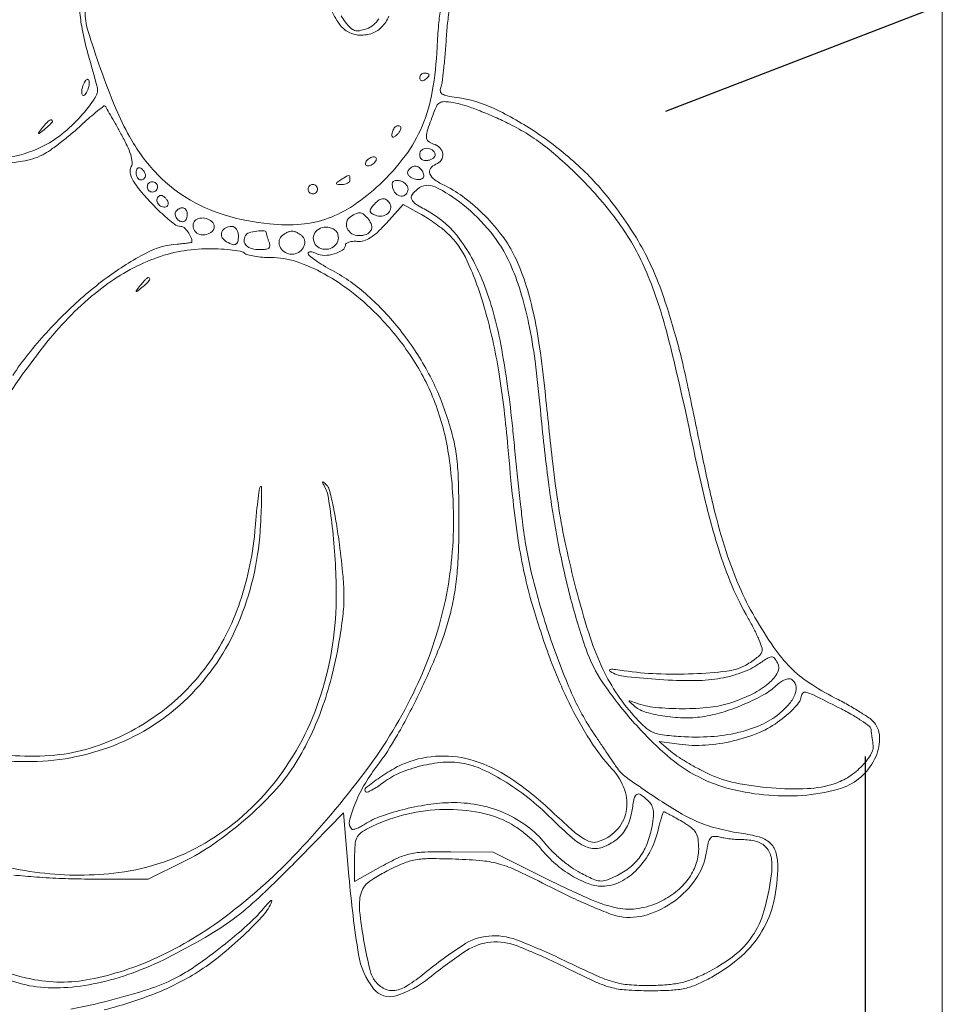
# Model space of a CAD drawing. Units: inches. Extents: x 2656 to 9931, y 1941 to 3068.
# Tile 35 of 46: x 2854 to 2868, y 2952 to 2967. Entities that reach past the tile are written whole.
import ezdxf

# ---------------------------------------------------------------- set-up
doc = ezdxf.new("R2010")
doc.units = ezdxf.units.IN
for name, color, linetype, lineweight in [('A-ANNO-DIMS', 2, 'Continuous', 18), ('A-ELEV-FNSH', 8, 'Continuous', 13), ('A-ELEV-ORN', 8, 'Continuous', 13)]:
    doc.layers.add(name, color=color, linetype=linetype, lineweight=lineweight)
doc.styles.get("Standard").update_dxf_attribs({"font": 'arial.ttf'})
doc.dimstyles.new('ISO-25', dxfattribs={"dimtxt": 6, "dimasz": 2.5, "dimexe": 1.25, "dimexo": 0.625, "dimtad": 1, "dimdec": 0, "dimlunit": 3, "dimtxsty": 'Standard', "dimcen": 2.5, "dimadec": 0, "dimazin": 0, "dimtfac": 1, "dimtdec": 0, "dimtmove": 0, "dimatfit": 3, "dimfxl": 1, "dimarcsym": 0})

# ---------------------------------------------------------------- blocks, each defined once
blk = doc.blocks.new('*D151')
at = {"layer": 'A-ANNO-DIMS', "color": 0, "lineweight": -2, "transparency": 16777216}
for p, q in [((2829.546, 2956.424), (2829.546, 2703.709)), ((2867.059, 2955.98), (2867.059, 2703.709)), ((2832.046, 2704.959), (2864.559, 2704.959))]:
    blk.add_line(p, q, dxfattribs=at)
at = {"layer": 'A-ANNO-DIMS', "color": 0, "transparency": 16777216}
for points in [[(2832.046, 2705.376), (2832.046, 2704.543), (2829.546, 2704.959)], [(2864.559, 2705.376), (2864.559, 2704.543), (2867.059, 2704.959)]]:
    blk.add_solid(points, dxfattribs=at)
at = {"layer": 'Defpoints', "color": 0, "transparency": 16777216}
for p in [(2829.546, 2957.049), (2867.059, 2956.605), (2867.059, 2704.959)]:
    blk.add_point(p, dxfattribs=at)
at = {"layer": 'A-ANNO-DIMS', "color": 0, "transparency": 16777216, "insert": (2848.302, 2708.689), "char_height": 6, "attachment_point": 5}
blk.add_mtext('3\'-1 1/2"', dxfattribs=at)
blk = doc.blocks.new('*D166')
at = {"layer": 'A-ANNO-DIMS', "color": 0, "lineweight": -2, "transparency": 16777216}
for p, q in [((2884.455, 2990.075), (2890.436, 2974.616)), ((2876.883, 2987.145), (2882.863, 2971.687)), ((2887.653, 2974.88), (2884.744, 2973.755)), ((2882.412, 2972.852), (2864.04, 2965.744))]:
    blk.add_line(p, q, dxfattribs=at)
at = {"layer": 'A-ANNO-DIMS', "color": 0, "transparency": 16777216}
for points in [[(2887.503, 2975.269), (2887.803, 2974.491), (2889.985, 2975.782)], [(2884.594, 2974.143), (2884.894, 2973.366), (2882.412, 2972.852)]]:
    blk.add_solid(points, dxfattribs=at)
at = {"layer": 'Defpoints', "color": 0, "transparency": 16777216}
for p in [(2884.229, 2990.658), (2876.657, 2987.728), (2882.412, 2972.852)]:
    blk.add_point(p, dxfattribs=at)
at = {"layer": 'A-ANNO-DIMS', "color": 0, "transparency": 16777216, "insert": (2870.73, 2972.287), "char_height": 6, "attachment_point": 5, "rotation": 21.1508}
blk.add_mtext('0\'-8"', dxfattribs=at)

msp = doc.modelspace()

# ---------------------------------------------------------------- linework, layer by layer
at = {"layer": 'A-ELEV-FNSH'}
msp.add_lwpolyline([(2826.64, 2994.347), (2868.226, 2994.347), (2868.226, 2892.035), (2826.64, 2892.035)], close=True, dxfattribs=at)
at = {"layer": 'A-ELEV-ORN'}
for points in [[(2855.174, 2967.3, 0.028596), (2855.206, 2967.037, 0.019917), (2855.288, 2966.67, 0.006616), (2855.436, 2966.14, -0.21756), (2855.409, 2965.955, -0.040075), (2855.195, 2965.675, -0.041303), (2854.904, 2965.4, -0.056735), (2854.6, 2965.209, -0.074881), (2854.055, 2965.042, -0.054125)], [(2854.109, 2952.6, 0.063438), (2854.524, 2952.497, 0.048495), (2854.996, 2952.487, 0.037857), (2855.505, 2952.565, 0.034879), (2856.037, 2952.728, 0.028198), (2856.582, 2952.973, 0.013653), (2857.141, 2953.284, 0.030316), (2857.545, 2953.557, 0.026779), (2857.942, 2953.897, 0.008593), (2858.495, 2954.443), (2859.166, 2955.13), (2859.249, 2954.169, 0.017456), (2859.394, 2952.984, 0.128416), (2859.621, 2952.466, 0.311108), (2859.962, 2952.36, 0.095606), (2860.463, 2952.63, -0.025392), (2861.026, 2953.043, -0.124698), (2861.396, 2953.172, -0.116398), (2861.795, 2953.114, -0.020849), (2862.488, 2952.806, 0.006689), (2862.954, 2952.582, 0.039752), (2863.207, 2952.488, 0.052181), (2863.442, 2952.448, 0.016514), (2863.798, 2952.436, 0.012108), (2864.123, 2952.444, 0.04207), (2864.331, 2952.472, 0.049914), (2864.513, 2952.531, 0.022452), (2864.737, 2952.643, 0.054702), (2865.187, 2952.96, 0.078378), (2865.497, 2953.336, 0.078505), (2865.676, 2953.788, 0.05507), (2865.736, 2954.334, 0.073105), (2865.706, 2954.537, 0.14057), (2865.618, 2954.674, 0.111241), (2865.454, 2954.764, 0.036328), (2865.182, 2954.82, -0.017364), (2865.028, 2954.846, -0.011942), (2864.854, 2954.885, -0.012054), (2864.69, 2954.932, -0.023906), (2864.562, 2954.978, -0.035914), (2864.252, 2955.133, -0.013112), (2863.836, 2955.395, -0.010281), (2863.442, 2955.67, -0.087803), (2863.294, 2955.825, 0.00053), (2863.245, 2955.897, 0.000109), (2863.16, 2956.023, 0.000114), (2863.061, 2956.171, 0.000108), (2862.959, 2956.321, -0.045796), (2862.618, 2956.942, -0.021393), (2862.287, 2957.8, -0.021231), (2862.02, 2958.719, -0.0319), (2861.874, 2959.54, -0.001287), (2861.841, 2959.838, -0.000643), (2861.801, 2960.214, -0.000639), (2861.76, 2960.604, -0.000943), (2861.726, 2960.947, 0.020553), (2861.546, 2962.22, 0.04686), (2861.284, 2963.153, 0.064624), (2860.927, 2963.81, 0.108526), (2860.461, 2964.226, -0.013252), (2860.262, 2964.345, -0.1368), (2860.198, 2964.415, -0.28166), (2860.204, 2964.483, -0.060529), (2860.288, 2964.572, -0.292683), (2860.552, 2964.604, -0.058258), (2860.972, 2964.339, -0.052773), (2861.394, 2963.918, -0.064866), (2861.686, 2963.444, -0.030734), (2861.844, 2963.023, -0.02351), (2861.967, 2962.546, -0.019015), (2862.065, 2961.967, -0.009465), (2862.146, 2961.228, 0.00962), (2862.266, 2960.142, 0.014652), (2862.416, 2959.206, 0.016506), (2862.603, 2958.374, 0.019831), (2862.836, 2957.606, 0.066026), (2863.091, 2957.098, 0.031307), (2863.541, 2956.518, 0.031311), (2864.062, 2955.996, 0.063647), (2864.54, 2955.672, 0.055485), (2865.032, 2955.488, 0.042522), (2865.599, 2955.395, 0.042331), (2866.177, 2955.399, 0.053334), (2866.701, 2955.504, 0.104768), (2866.992, 2955.669, 0.096785), (2867.202, 2955.942, 0.109583), (2867.278, 2956.245, 0.172667), (2867.195, 2956.497, 0.078073), (2867.133, 2956.555, 0.010534), (2866.983, 2956.654, 0.01194), (2866.799, 2956.763, 0.009802), (2866.597, 2956.871, -0.028546), (2866.213, 2957.096, -0.050975), (2865.93, 2957.328, -0.045238), (2865.679, 2957.631, -0.017925), (2865.39, 2958.088, -0.030624), (2865.156, 2958.552, -0.023473), (2864.956, 2959.083, -0.018746), (2864.771, 2959.74, -0.008967), (2864.581, 2960.595, 0.001102), (2864.391, 2961.515, 0.006759), (2864.285, 2961.988, 0.011262), (2864.191, 2962.348, 0.007165), (2864.067, 2962.762, 0.018233), (2863.907, 2963.21, 0.025477), (2863.729, 2963.597, 0.025141), (2863.511, 2963.968, 0.017087), (2863.228, 2964.368, 0.044384), (2862.72, 2964.925, 0.037111), (2862.093, 2965.421, 0.038623), (2861.444, 2965.79, 0.076899), (2860.879, 2965.957, -0.016318), (2860.734, 2965.981, -0.091012), (2860.661, 2966.01, -0.208145), (2860.633, 2966.051, -0.140788), (2860.638, 2966.109, 0.059531), (2860.657, 2966.183, 0.005389), (2860.681, 2966.375, 0.006933), (2860.703, 2966.604, 0.005366), (2860.722, 2966.855, -0.012637), (2860.744, 2967.112, -0.013655), (2860.78, 2967.361, -0.013252)], [(2860.639, 2967.314, 0.023375), (2860.606, 2967.062, 0.009261), (2860.583, 2966.714, -0.031116), (2860.51, 2966.049, -0.056426), (2860.356, 2965.523, -0.061102), (2860.1, 2965.074, -0.043729), (2859.714, 2964.642, -0.039093), (2859.318, 2964.324, -0.06347), (2858.935, 2964.129, -0.065711), (2858.524, 2964.039, -0.045332), (2858.048, 2964.043, -0.049376), (2857.363, 2964.18, -0.065569), (2856.785, 2964.443, -0.067894), (2856.31, 2964.838, -0.058197), (2855.929, 2965.366, -0.029232), (2855.719, 2965.799, -0.012926), (2855.492, 2966.391, -0.010579), (2855.3, 2966.971, -0.074704), (2855.256, 2967.264, -0.0517)], [(2858.97, 2967.304, 0.041294), (2859.105, 2967.067, 0.109032), (2859.227, 2966.955, 0.109354), (2859.384, 2966.903, 0.099066), (2859.581, 2966.923, 0.120027), (2859.739, 2967.018, 0.102309), (2859.854, 2967.189, 0.057096)], [(2859.7, 2967.146, -0.082559), (2859.62, 2967.056, -0.084337), (2859.515, 2966.998, -0.038037), (2859.407, 2966.968, -0.127103), (2859.335, 2966.973, -0.11952), (2859.271, 2967.012, -0.031788), (2859.191, 2967.103, -0.033217), (2859.132, 2967.192, -0.013391)], [(2853.796, 2964.937, 0.021823), (2854.311, 2964.991, 0.083985), (2854.616, 2965.091, 0.031152), (2854.732, 2965.161, 0.011426), (2854.886, 2965.274, 0.011275), (2855.049, 2965.405, 0.013273), (2855.198, 2965.537, -0.007108), (2855.33, 2965.657, -0.011939), (2855.446, 2965.754, -0.005638), (2855.543, 2965.83, -0.413391), (2855.561, 2965.828, -0.034188), (2855.576, 2965.806, -0.000712), (2855.64, 2965.693, -0.001658), (2855.715, 2965.561, -0.001115), (2855.799, 2965.409, -0.014931), (2855.892, 2965.228, -0.035606), (2855.947, 2965.088, -0.049197), (2855.97, 2964.981, -0.155471), (2855.955, 2964.911, 0.120552), (2855.939, 2964.851, 0.082364), (2855.948, 2964.78, 0.06067), (2855.985, 2964.698, 0.029026), (2856.05, 2964.602, 0.022485), (2856.228, 2964.391, 0.021702), (2856.426, 2964.195, 0.01756), (2856.61, 2964.039, 0.16831), (2856.706, 2964.006, -0.187338), (2856.757, 2963.987, -0.053599), (2856.814, 2963.922, -0.052999), (2856.859, 2963.842, -0.101355), (2856.874, 2963.769, -0.369146), (2856.868, 2963.763, -0.003978), (2856.808, 2963.754, -0.010014), (2856.737, 2963.745, -0.006066), (2856.652, 2963.738, 0.102377), (2856.179, 2963.602, 0.038016), (2855.589, 2963.232, 0.034625), (2854.97, 2962.705, 0.029805), (2854.396, 2962.072, 0.025999), (2854.163, 2961.749, 0.003163)], [(2853.875, 2961.115, -0.028373), (2854.681, 2962.254, -0.056082), (2855.463, 2963.036, -0.071786), (2856.251, 2963.498, -0.092393), (2857.071, 2963.666, -0.013431), (2857.27, 2963.665, -0.017308), (2857.452, 2963.652, -0.015196), (2857.601, 2963.632, -0.126503), (2857.663, 2963.604, 0.101758), (2857.717, 2963.577, 0.023151), (2857.819, 2963.554, 0.023036), (2857.942, 2963.539, 0.020609), (2858.069, 2963.534, -0.081277), (2858.449, 2963.474, -0.046227), (2858.875, 2963.287, -0.041516), (2859.312, 2962.996, -0.034768), (2859.724, 2962.62, -0.047065), (2860.226, 2961.981, -0.056002), (2860.567, 2961.294, -0.052207), (2860.763, 2960.51, -0.033786), (2860.831, 2959.575, -0.05658), (2860.69, 2958.266, -0.055783), (2860.258, 2957.014, -0.04941), (2859.505, 2955.766, -0.030886), (2858.401, 2954.463, -0.039889), (2857.397, 2953.571, -0.052556), (2856.348, 2952.94, -0.060616), (2855.335, 2952.61, -0.099916), (2854.437, 2952.614, -0.051733), (2853.786, 2952.82, -0.039695)], [(2854.178, 2954.187, 0.008256), (2854.522, 2954.157, 0.008262), (2854.912, 2954.135, 0.008791), (2855.295, 2954.127), (2856.213, 2954.124), (2856.741, 2954.385, 0.037754), (2857.203, 2954.659, 0.026153), (2857.682, 2955.032, 0.026418), (2858.109, 2955.444, 0.045079), (2858.414, 2955.836, 0.028905), (2858.644, 2956.245, 0.02616), (2858.835, 2956.692, 0.024873), (2858.985, 2957.179, 0.020872), (2859.098, 2957.707, 0.011221), (2859.156, 2958.106, 0.029314), (2859.174, 2958.396, 0.025822), (2859.16, 2958.705, 0.00712), (2859.105, 2959.189, 0.00881), (2859.059, 2959.509, 0.012431), (2859.006, 2959.792, 0.008644), (2858.952, 2960.024, 0.14575), (2858.912, 2960.091, 0.005212), (2858.864, 2960.133, 0.236159), (2858.852, 2960.137, 0.498193), (2858.848, 2960.129, 0.008614), (2858.874, 2960.083, -0.089875), (2858.939, 2959.894, -0.011245), (2858.997, 2959.464, -0.013414), (2859.04, 2958.961, -0.012898), (2859.057, 2958.45, -0.078199), (2858.825, 2956.917, -0.089178), (2858.136, 2955.605, -0.094631), (2857.073, 2954.672, -0.101406), (2855.766, 2954.225, -0.06271), (2854.574, 2954.222, -0.059511), (2853.396, 2954.512, -0.061335)], [(2854.024, 2955.915, 0.013073), (2854.359, 2955.904, 0.095042), (2855.696, 2956.15, 0.101899), (2856.811, 2956.872, 0.098684), (2857.574, 2957.997, 0.08367), (2857.906, 2959.398, 0.004935), (2857.92, 2959.655, 0.008259), (2857.927, 2959.871, 0.002726), (2857.928, 2960.054, 0.414775), (2857.915, 2960.068, 0.371773), (2857.899, 2960.054, 0.003199), (2857.876, 2959.889, 0.008961), (2857.853, 2959.692, 0.005421), (2857.832, 2959.459, -0.062277), (2857.6, 2958.319, -0.076581), (2857.101, 2957.356, -0.079646), (2856.354, 2956.616, -0.0747), (2855.397, 2956.127, -0.053032), (2854.872, 2956.011, -0.038092), (2854.272, 2955.99, -0.038832), (2853.696, 2956.059, -0.070977)], [(2855.548, 2952.148, 0.033055), (2856.284, 2952.381, 0.043026), (2856.918, 2952.694, 0.031455), (2857.248, 2952.924, 0.018917), (2857.611, 2953.235, 0.017394), (2857.928, 2953.549, 0.078159), (2858.074, 2953.763, 0.114181), (2858.081, 2953.795, 0.599459), (2858.069, 2953.802, 0.059878), (2858.025, 2953.763, 0.010894), (2857.955, 2953.682, -0.039265), (2857.711, 2953.427, -0.0147), (2857.331, 2953.109, -0.014829), (2856.93, 2952.811, -0.035002), (2856.61, 2952.62, -0.03988), (2856.209, 2952.456, -0.015079), (2855.626, 2952.288, -0.01477), (2855.041, 2952.158, -0.047431)]]:
    msp.add_lwpolyline(points, format="xyb", dxfattribs=at)
for points in [[(2855.228, 2966.144, 0.033304), (2855.213, 2966.096, 0.041541), (2855.206, 2966.05, 0.04665), (2855.207, 2966.012, 0.168083), (2855.218, 2965.991, 0.291964), (2855.235, 2965.987, 0.11331), (2855.256, 2966.001, 0.066301), (2855.278, 2966.031, 0.03436), (2855.298, 2966.074, 0.033304), (2855.313, 2966.122, 0.041541), (2855.32, 2966.168, 0.04665), (2855.319, 2966.206, 0.168083), (2855.309, 2966.228, 0.291964), (2855.292, 2966.232, 0.11331), (2855.27, 2966.218, 0.066301), (2855.248, 2966.187, 0.03436)], [(2860.32, 2966.253, 0.108972), (2860.326, 2966.228, 0.182303), (2860.341, 2966.213, 0.161196), (2860.364, 2966.211, 0.082592), (2860.39, 2966.222, 0.029505), (2860.417, 2966.241, 0.035638), (2860.44, 2966.262, 0.038439), (2860.456, 2966.282, 0.151918), (2860.461, 2966.296, 0.210953), (2860.456, 2966.308, 0.081139), (2860.44, 2966.318, 0.061769), (2860.417, 2966.325, 0.042167), (2860.39, 2966.327, 0.105053), (2860.364, 2966.322, 0.099167), (2860.341, 2966.305, 0.09642), (2860.325, 2966.281, 0.093332)], [(2861.648, 2965.571, -0.02318), (2861.924, 2965.42, -0.024394), (2862.179, 2965.246, -0.021618), (2862.441, 2965.03, -0.012473), (2862.739, 2964.749, -0.039784), (2863.327, 2964.063, -0.054855), (2863.73, 2963.359, -0.039702), (2864.051, 2962.425, -0.011344), (2864.399, 2960.931, 0.006591), (2864.634, 2959.877, 0.017333), (2864.839, 2959.13, 0.02365), (2865.047, 2958.558, 0.033029), (2865.29, 2958.071, -0.014848), (2865.38, 2957.905, -0.020336), (2865.451, 2957.751, -0.017573), (2865.498, 2957.622, -0.172671), (2865.497, 2957.564, -0.10754), (2865.469, 2957.521, -0.026105), (2865.405, 2957.465, -0.025574), (2865.322, 2957.406, -0.022994), (2865.232, 2957.354, -0.091881), (2864.964, 2957.273, -0.017748), (2864.458, 2957.234, -0.019702), (2863.902, 2957.234, -0.028696), (2863.415, 2957.281, 0.009481), (2863.282, 2957.299, 0.047771), (2863.208, 2957.301, 0.368655), (2863.193, 2957.286, 0.282694), (2863.204, 2957.266, 0.108907), (2863.401, 2957.197, 0.011453), (2863.888, 2957.151, 0.015255), (2864.397, 2957.13, 0.03383), (2864.785, 2957.152, 0.026779), (2864.958, 2957.183, 0.023197), (2865.136, 2957.233, 0.024046), (2865.297, 2957.296, 0.044005), (2865.421, 2957.365, -0.008574), (2865.576, 2957.467, -0.115161), (2865.64, 2957.489, -0.24786), (2865.685, 2957.47, -0.052764), (2865.734, 2957.398, -0.252743), (2865.734, 2957.255, -0.09163), (2865.602, 2957.092, -0.061736), (2865.357, 2956.931, -0.0348), (2865.029, 2956.796, -0.05395), (2864.712, 2956.727, -0.025613), (2864.295, 2956.705, -0.025459), (2863.884, 2956.725, -0.063366), (2863.591, 2956.792, 0.002665), (2863.497, 2956.826, 0.435273), (2863.489, 2956.821, 0.294359), (2863.492, 2956.809, 0.002046), (2863.576, 2956.74, 0.103408), (2863.748, 2956.65, 0.033459), (2864.03, 2956.59, 0.033234), (2864.345, 2956.567, 0.044104), (2864.631, 2956.589, 0.034871), (2864.924, 2956.66, 0.024911), (2865.24, 2956.778, 0.025154), (2865.525, 2956.918, 0.061455), (2865.713, 2957.055, -0.038429), (2865.777, 2957.107, -0.049791), (2865.843, 2957.143, -0.058947), (2865.902, 2957.16, -0.181439), (2865.942, 2957.152, -0.197915), (2866.008, 2957.061, -0.144406), (2866.001, 2956.935, -0.091074), (2865.915, 2956.784, -0.045063), (2865.758, 2956.629, -0.069066), (2865.483, 2956.46, -0.046466), (2865.133, 2956.343, -0.04134), (2864.724, 2956.283, -0.031546), (2864.271, 2956.284, -0.014263), (2863.992, 2956.309, -0.074232), (2863.843, 2956.35, -0.085177), (2863.723, 2956.43, -0.022019), (2863.56, 2956.598, -0.037141), (2863.284, 2956.96, -0.037651), (2863.066, 2957.357, -0.030309), (2862.876, 2957.853, -0.01342), (2862.683, 2958.526, -0.009543), (2862.531, 2959.17, -0.014589), (2862.425, 2959.734, -0.010692), (2862.333, 2960.417, -0.002836), (2862.216, 2961.509, 0.010339), (2862.134, 2962.178, 0.01936), (2862.036, 2962.714, 0.023505), (2861.914, 2963.159, 0.031963), (2861.76, 2963.546, 0.049968), (2861.575, 2963.854, 0.0337), (2861.308, 2964.165, 0.033863), (2861.004, 2964.435, 0.053574), (2860.708, 2964.618, -0.041158), (2860.548, 2964.711, -0.139511), (2860.473, 2964.803, -0.269863), (2860.483, 2964.883, -0.140125), (2860.566, 2964.946, 0.157607), (2860.645, 2965.01, 0.176741), (2860.668, 2965.105, 0.164098), (2860.624, 2965.197, 0.136791), (2860.529, 2965.252, -0.116926), (2860.45, 2965.295, -0.222136), (2860.421, 2965.36, -0.076329), (2860.442, 2965.477, -0.007145), (2860.542, 2965.755, -0.052374), (2860.586, 2965.844, -0.164893), (2860.637, 2965.885, -0.113688), (2860.715, 2965.894, -0.018928), (2860.866, 2965.873, -0.036795), (2861.001, 2965.838, -0.010627), (2861.204, 2965.765, -0.010627), (2861.43, 2965.672, -0.011143)], [(2854.614, 2965.501, 0.001576), (2854.552, 2965.421, 0.377591), (2854.553, 2965.413, 0.377591), (2854.561, 2965.412, 0.001576), (2854.641, 2965.474, 0.012436), (2854.688, 2965.513, 0.017649), (2854.728, 2965.55, 0.013803), (2854.758, 2965.583, 0.184603), (2854.764, 2965.597, 0.307699), (2854.75, 2965.617, 0.241985), (2854.723, 2965.615, 0.065617), (2854.677, 2965.575, 0.017685)], [(2859.945, 2965.507, 0.063896), (2859.927, 2965.484, 0.039129), (2859.912, 2965.452, 0.038674), (2859.902, 2965.418, 0.054831), (2859.898, 2965.387, 0.142677), (2859.905, 2965.365, 0.290264), (2859.921, 2965.357, 0.131573), (2859.947, 2965.368, 0.034019), (2859.981, 2965.398, 0.041736), (2860.011, 2965.432, 0.061283), (2860.029, 2965.467, 0.080535), (2860.036, 2965.497, 0.212536), (2860.028, 2965.517, 0.128169), (2860.011, 2965.528, 0.100736), (2859.989, 2965.529, 0.089268), (2859.966, 2965.522, 0.075941)], [(2860.552, 2965.097, -0.173043), (2860.548, 2965.069, -0.094518), (2860.526, 2965.041, -0.074555), (2860.489, 2965.019, -0.054517), (2860.443, 2965.004, -0.075042), (2860.392, 2965.002, -0.134068), (2860.353, 2965.018, -0.143006), (2860.329, 2965.05, -0.090288), (2860.32, 2965.096, -0.226436), (2860.351, 2965.162, -0.170609), (2860.427, 2965.189, -0.153586), (2860.509, 2965.163, -0.194407)], [(2859.511, 2964.991, 0.076764), (2859.5, 2964.964, 0.154201), (2859.501, 2964.941, 0.186277), (2859.515, 2964.926, 0.117858), (2859.538, 2964.921, 0.085235), (2859.568, 2964.926, 0.053414), (2859.601, 2964.941, 0.051777), (2859.63, 2964.964, 0.064269), (2859.652, 2964.991, 0.076764), (2859.663, 2965.018, 0.154201), (2859.662, 2965.041, 0.186277), (2859.648, 2965.056, 0.117858), (2859.625, 2965.061, 0.085235), (2859.595, 2965.056, 0.053414), (2859.563, 2965.041, 0.051777), (2859.533, 2965.018, 0.064269)], [(2856.17, 2964.776, -0.105429), (2856.165, 2964.751, -0.099231), (2856.15, 2964.729, -0.096318), (2856.127, 2964.715, -0.092995), (2856.1, 2964.71, -0.153634), (2856.073, 2964.718, -0.097988), (2856.05, 2964.742, -0.080552), (2856.035, 2964.777, -0.062283), (2856.03, 2964.819, -0.066118), (2856.035, 2964.858, -0.138808), (2856.05, 2964.884, -0.191142), (2856.073, 2964.893, -0.139169), (2856.1, 2964.885, -0.06081), (2856.127, 2964.864, -0.051032), (2856.15, 2964.835, -0.053229), (2856.165, 2964.804, -0.089642)], [(2860.358, 2964.846, -0.113371), (2860.381, 2964.779, -0.261672), (2860.36, 2964.732, -0.188422), (2860.301, 2964.715, -0.067736), (2860.213, 2964.736, -0.067341), (2860.173, 2964.757, -0.097937), (2860.146, 2964.787, -0.123144), (2860.136, 2964.819, -0.153283), (2860.144, 2964.85, -0.104938), (2860.192, 2964.9, -0.155876), (2860.251, 2964.918, -0.152164), (2860.309, 2964.898, -0.098738)], [(2859.124, 2964.71, 0.011213), (2859.066, 2964.67, 0.309569), (2859.06, 2964.654, 0.327416), (2859.073, 2964.643, 0.011938), (2859.142, 2964.64, 0.055234), (2859.189, 2964.645, 0.075283), (2859.229, 2964.66, 0.095191), (2859.256, 2964.683, 0.17131), (2859.265, 2964.71, 0.042895), (2859.261, 2964.76, 0.364836), (2859.245, 2964.774, 0.137048), (2859.213, 2964.765, 0.007234)], [(2856.342, 2964.563, -0.099038), (2856.322, 2964.541, -0.097945), (2856.294, 2964.528, -0.097945), (2856.263, 2964.527, -0.099038), (2856.235, 2964.538, -0.099038), (2856.212, 2964.558, -0.097945), (2856.2, 2964.586, -0.097945), (2856.199, 2964.617, -0.099038), (2856.209, 2964.645, -0.099038), (2856.23, 2964.668, -0.097945), (2856.258, 2964.68, -0.097945), (2856.288, 2964.681, -0.099038), (2856.317, 2964.671, -0.099038), (2856.339, 2964.65, -0.097945), (2856.352, 2964.622, -0.097945), (2856.353, 2964.592, -0.099038)], [(2858.632, 2964.569, 0.099038), (2858.637, 2964.542, 0.097945), (2858.653, 2964.519, 0.097945), (2858.676, 2964.504, 0.099038), (2858.702, 2964.499, 0.099038), (2858.729, 2964.504, 0.097945), (2858.752, 2964.519, 0.097945), (2858.767, 2964.542, 0.099038), (2858.773, 2964.569, 0.099038), (2858.767, 2964.596, 0.097945), (2858.752, 2964.619, 0.097945), (2858.729, 2964.634, 0.099038), (2858.702, 2964.639, 0.099038), (2858.676, 2964.634, 0.097945), (2858.653, 2964.619, 0.097945), (2858.637, 2964.596, 0.099038)], [(2860.144, 2964.568, -0.200576), (2860.113, 2964.492, -0.224971), (2860.038, 2964.466, -0.174236), (2859.956, 2964.506, -0.147142), (2859.91, 2964.593, -0.055061), (2859.905, 2964.652, -0.191187), (2859.92, 2964.687, -0.191187), (2859.955, 2964.702, -0.055061), (2860.015, 2964.697, -0.073891), (2860.064, 2964.68, -0.07517), (2860.106, 2964.649, -0.081554), (2860.134, 2964.61, -0.115485)], [(2856.504, 2964.317, -0.222509), (2856.449, 2964.297, -0.14837), (2856.385, 2964.323, -0.146836), (2856.346, 2964.38, -0.218805), (2856.353, 2964.439, -0.094625), (2856.377, 2964.466, -0.169261), (2856.405, 2964.474, -0.136091), (2856.437, 2964.465, -0.053431), (2856.473, 2964.436, -0.055675), (2856.498, 2964.404, -0.075207), (2856.513, 2964.37, -0.09457), (2856.515, 2964.339, -0.169316)], [(2860.726, 2963.916, -0.101297), (2861.04, 2963.479, -0.035873), (2861.305, 2962.752, -0.030071), (2861.515, 2961.806, -0.018203), (2861.654, 2960.665, 0.005327), (2861.731, 2959.86, 0.011878), (2861.811, 2959.249, 0.014991), (2861.905, 2958.744, 0.017814), (2862.025, 2958.274, 0.017182), (2862.288, 2957.476, 0.024765), (2862.58, 2956.792, 0.028345), (2862.896, 2956.228, 0.045869), (2863.232, 2955.792, -0.105006), (2863.419, 2955.48, -0.132887), (2863.442, 2955.145, -0.143146), (2863.294, 2954.862, -0.129359), (2863.011, 2954.69, -0.148432), (2862.906, 2954.69, -0.071268), (2862.782, 2954.749, -0.036276), (2862.611, 2954.881, -0.007236), (2862.326, 2955.143, 0.036242), (2861.745, 2955.618, 0.067997), (2861.206, 2955.897, 0.082598), (2860.689, 2955.989, 0.083918), (2860.172, 2955.908, 0.045356), (2859.96, 2955.815, 0.024688), (2859.717, 2955.665, 0.01659), (2859.506, 2955.508, 0.448591), (2859.502, 2955.446, 0.305983), (2859.527, 2955.442, 0.021853), (2859.596, 2955.474, 0.024798), (2859.679, 2955.524, 0.015673), (2859.772, 2955.59, -0.063533), (2860.019, 2955.733, -0.038947), (2860.338, 2955.839, -0.038947), (2860.67, 2955.894, -0.063525), (2860.955, 2955.882, -0.065258), (2861.266, 2955.787, -0.033299), (2861.626, 2955.593, -0.030456), (2862, 2955.324, -0.026779), (2862.356, 2955.001, 0.023706), (2862.667, 2954.717, 0.1035), (2862.885, 2954.6, 0.158338), (2863.082, 2954.606, 0.080448), (2863.3, 2954.727, 0.053384), (2863.382, 2954.808, 0.04826), (2863.449, 2954.906, 0.045818), (2863.498, 2955.021, 0.039107), (2863.529, 2955.149, -0.012003), (2863.566, 2955.35, -0.189821), (2863.604, 2955.407, -0.317878), (2863.658, 2955.407, -0.02959), (2863.769, 2955.318, -0.073348), (2863.824, 2955.251, -0.091866), (2863.852, 2955.175, -0.066858), (2863.857, 2955.077, -0.022444), (2863.837, 2954.934, -0.045022), (2863.766, 2954.677, -0.063757), (2863.655, 2954.468, -0.067774), (2863.5, 2954.303, -0.059979), (2863.301, 2954.177, -0.023864), (2863.144, 2954.111, -0.107712), (2863.046, 2954.098, -0.088854), (2862.942, 2954.125, -0.013401), (2862.749, 2954.221, -0.032881), (2862.616, 2954.303, -0.019147), (2862.467, 2954.418, -0.019089), (2862.326, 2954.545, -0.030435), (2862.217, 2954.666, 0.062264), (2861.95, 2954.923, 0.055565), (2861.619, 2955.119, 0.053876), (2861.243, 2955.242, 0.051591), (2860.843, 2955.284, 0.034546), (2860.488, 2955.26, 0.025142), (2860.099, 2955.187, 0.025521), (2859.741, 2955.081, 0.057544), (2859.488, 2954.957, -0.022338), (2859.422, 2954.919, -0.033258), (2859.362, 2954.892, -0.035169), (2859.312, 2954.878, -0.253082), (2859.29, 2954.885, -0.260885), (2859.257, 2955.002, -0.035632), (2859.336, 2955.253, -0.035977), (2859.476, 2955.543, -0.032126), (2859.662, 2955.822, 0.033509), (2859.982, 2956.308, 0.017139), (2860.32, 2956.955, 0.017135), (2860.613, 2957.622, 0.034444), (2860.788, 2958.169, 0.021084), (2860.849, 2958.47, 0.018217), (2860.888, 2958.79, 0.014973), (2860.908, 2959.167, 0.007448), (2860.913, 2959.646, 0.006272), (2860.903, 2960.19, 0.023889), (2860.876, 2960.529, 0.031276), (2860.822, 2960.815, 0.017227), (2860.721, 2961.158, 0.045426), (2860.433, 2961.82, 0.041706), (2860.022, 2962.439, 0.043013), (2859.531, 2962.962, 0.058194), (2859.001, 2963.336, -0.012033), (2858.86, 2963.417, -0.017924), (2858.741, 2963.495, -0.013179), (2858.648, 2963.565, -0.228958), (2858.632, 2963.598, -0.264434), (2858.642, 2963.616, -0.140927), (2858.668, 2963.623, -0.077634), (2858.708, 2963.616, -0.037384), (2858.755, 2963.595, 0.125259), (2858.875, 2963.567, 0.066377), (2859.027, 2963.589, 0.071856), (2859.153, 2963.647, 0.256135), (2859.195, 2963.722, -0.238209), (2859.208, 2963.748, -0.081837), (2859.247, 2963.768, -0.059758), (2859.305, 2963.779, -0.038169), (2859.373, 2963.779, 0.090703), (2859.472, 2963.789, 0.069319), (2859.57, 2963.832, 0.04998), (2859.68, 2963.916, 0.020141), (2859.811, 2964.051), (2860.07, 2964.338), (2860.318, 2964.2, -0.015106), (2860.425, 2964.137, -0.010818), (2860.54, 2964.06, -0.010939), (2860.647, 2963.982, -0.022966)], [(2859.867, 2964.352, -0.196524), (2859.88, 2964.273, -0.167237), (2859.835, 2964.201, -0.136751), (2859.747, 2964.163, -0.127721), (2859.649, 2964.174, -0.043397), (2859.591, 2964.202, -0.209307), (2859.571, 2964.231, -0.191145), (2859.577, 2964.267, -0.035728), (2859.617, 2964.324, -0.049461), (2859.691, 2964.396, -0.142888), (2859.756, 2964.424, -0.188214), (2859.815, 2964.408, -0.096738)], [(2856.803, 2964.182, -0.06085), (2856.798, 2964.142, -0.079459), (2856.784, 2964.108, -0.097386), (2856.762, 2964.085, -0.156819), (2856.737, 2964.077, -0.139398), (2856.679, 2964.093, -0.123736), (2856.635, 2964.139, -0.139481), (2856.621, 2964.195, -0.191124), (2856.641, 2964.243, -0.094876), (2856.698, 2964.282, -0.1934), (2856.752, 2964.283, -0.202875), (2856.79, 2964.247, -0.103624)], [(2859.544, 2964.115, -0.109195), (2859.591, 2964.024, -0.19828), (2859.58, 2963.942, -0.176707), (2859.512, 2963.885, -0.086689), (2859.399, 2963.866, -0.139486), (2859.292, 2963.896, -0.151227), (2859.222, 2963.978, -0.174991), (2859.215, 2964.076, -0.184411), (2859.272, 2964.153, -0.0339), (2859.362, 2964.202, -0.143064), (2859.422, 2964.21, -0.148362), (2859.476, 2964.185, -0.037379)], [(2857.208, 2964.024, -0.249378), (2857.195, 2963.949, -0.140064), (2857.119, 2963.893, -0.117741), (2857.015, 2963.88, -0.170266), (2856.931, 2963.921, -0.08302), (2856.907, 2963.955, -0.075174), (2856.894, 2963.996, -0.077648), (2856.894, 2964.038, -0.099717), (2856.907, 2964.074, -0.179958), (2856.972, 2964.124, -0.118434), (2857.066, 2964.131, -0.113816), (2857.156, 2964.094, -0.158698)], [(2857.577, 2963.866, -0.056091), (2857.567, 2963.774, -0.250731), (2857.532, 2963.734, -0.198442), (2857.473, 2963.736, -0.036271), (2857.375, 2963.789, -0.164496), (2857.325, 2963.85, -0.199738), (2857.328, 2963.924, -0.166413), (2857.385, 2963.984, -0.119732), (2857.476, 2964.006, -0.137622), (2857.514, 2963.995, -0.100183), (2857.547, 2963.965, -0.086062), (2857.569, 2963.919, -0.070352)], [(2859.089, 2963.831, -0.170798), (2859.055, 2963.735, -0.139506), (2858.966, 2963.671, -0.132728), (2858.852, 2963.663, -0.150435), (2858.756, 2963.714, -0.167697), (2858.711, 2963.807, -0.171329), (2858.733, 2963.907, -0.154416), (2858.817, 2963.979, -0.136105), (2858.931, 2963.994, -0.062873), (2858.999, 2963.975, -0.10149), (2859.049, 2963.941, -0.11006), (2859.079, 2963.893, -0.084079)], [(2857.999, 2963.907, 0.065182), (2858.001, 2963.889, 0.008575), (2858.012, 2963.853, 0.009838), (2858.025, 2963.811, 0.008099), (2858.042, 2963.766, -0.088362), (2858.052, 2963.713, -0.229108), (2858.036, 2963.679, -0.141719), (2857.991, 2963.66, -0.030174), (2857.905, 2963.655, -0.062105), (2857.781, 2963.67, -0.128293), (2857.695, 2963.717, -0.188442), (2857.663, 2963.786, -0.156473), (2857.683, 2963.866, -0.181774), (2857.738, 2963.909, -0.042377), (2857.856, 2963.934, -0.044202), (2857.968, 2963.939, -0.400188)], [(2858.546, 2963.853, -0.186847), (2858.581, 2963.775, -0.146911), (2858.558, 2963.683, -0.127978), (2858.485, 2963.611, -0.131936), (2858.386, 2963.584, -0.131936), (2858.287, 2963.611, -0.127978), (2858.214, 2963.683, -0.146911), (2858.191, 2963.775, -0.186847), (2858.226, 2963.853, -0.041266), (2858.263, 2963.885, -0.035885), (2858.307, 2963.912, -0.037549), (2858.35, 2963.93, -0.081888), (2858.386, 2963.936, -0.081888), (2858.421, 2963.93, -0.037549), (2858.465, 2963.912, -0.035885), (2858.509, 2963.885, -0.041266)], [(2856.091, 2963.11, 0.001576), (2856.029, 2963.03, 0.377591), (2856.03, 2963.022, 0.377591), (2856.038, 2963.021, 0.001576), (2856.118, 2963.083, 0.017685), (2856.192, 2963.146, 0.065617), (2856.232, 2963.192, 0.241985), (2856.234, 2963.219, 0.307699), (2856.214, 2963.233, 0.184603), (2856.199, 2963.227, 0.013803), (2856.167, 2963.196, 0.017649), (2856.13, 2963.157, 0.012436)], [(2866.652, 2956.726, -0.012797), (2866.84, 2956.625, -0.018775), (2867, 2956.526, -0.014458), (2867.124, 2956.437, -0.217962), (2867.148, 2956.392, 0.013161), (2867.152, 2956.35, 0.005641), (2867.159, 2956.294, 0.005577), (2867.168, 2956.234, 0.007322), (2867.177, 2956.18, -0.177908), (2867.152, 2956.026, -0.062451), (2867.016, 2955.844, -0.056926), (2866.816, 2955.678, -0.064934), (2866.591, 2955.57, -0.06912), (2866.186, 2955.496, -0.0307), (2865.642, 2955.506, -0.030736), (2865.096, 2955.584, -0.06069), (2864.681, 2955.723, -0.012335), (2864.52, 2955.805, -0.010859), (2864.356, 2955.898, -0.010976), (2864.212, 2955.988, -0.032055), (2864.118, 2956.059), (2863.942, 2956.21), (2864.245, 2956.168, 0.051279), (2864.641, 2956.154, 0.040987), (2865.064, 2956.217, 0.041876), (2865.458, 2956.345, 0.063654), (2865.77, 2956.526, 0.018873), (2865.892, 2956.626, 0.024737), (2865.994, 2956.727, 0.023655), (2866.069, 2956.817, 0.163859), (2866.088, 2956.871, -0.158913), (2866.109, 2956.937, -0.307009), (2866.16, 2956.956, -0.051479), (2866.277, 2956.913, -0.002425)], [(2861.638, 2954.995, -0.036147), (2861.771, 2954.919, -0.020982), (2861.92, 2954.808, -0.020899), (2862.061, 2954.685, -0.032848), (2862.169, 2954.566, 0.046139), (2862.373, 2954.356, 0.041941), (2862.618, 2954.179, 0.04446), (2862.866, 2954.058, 0.091763), (2863.078, 2954.019, 0.116877), (2863.355, 2954.085, 0.084769), (2863.611, 2954.274, 0.075176), (2863.815, 2954.563, 0.063397), (2863.939, 2954.916, -0.010012), (2863.96, 2955.003, -0.016008), (2863.982, 2955.077, -0.009951), (2864.002, 2955.136, -0.313397), (2864.014, 2955.144, -0.120523), (2864.032, 2955.14, -0.002933), (2864.106, 2955.101, -0.006216), (2864.192, 2955.053, -0.004168), (2864.29, 2954.997, -0.027533), (2864.426, 2954.906, -0.09701), (2864.497, 2954.828, -0.102671), (2864.53, 2954.732, -0.032903), (2864.54, 2954.58, -0.086888), (2864.499, 2954.347, -0.0725), (2864.381, 2954.126, -0.066824), (2864.193, 2953.932, -0.056224), (2863.95, 2953.781, -0.072136), (2863.63, 2953.682, -0.086932), (2863.316, 2953.688, -0.054854), (2862.921, 2953.811, -0.01327), (2862.3, 2954.101), (2861.432, 2954.536), (2860.788, 2954.54, 0.00906), (2860.397, 2954.535, 0.045081), (2860.179, 2954.509, 0.056498), (2859.993, 2954.446, 0.019383), (2859.739, 2954.316), (2859.335, 2954.088), (2859.335, 2954.438, -0.016342), (2859.342, 2954.644, -0.091033), (2859.369, 2954.75, -0.124739), (2859.428, 2954.824, -0.04219), (2859.545, 2954.897, -0.056412), (2860.058, 2955.093, -0.05128), (2860.619, 2955.178, -0.052955), (2861.166, 2955.145, -0.071653)], [(2865.221, 2954.723, -0.077833), (2865.436, 2954.688, -0.15293), (2865.576, 2954.589, -0.138203), (2865.643, 2954.419, -0.058984), (2865.638, 2954.173, -0.035758), (2865.526, 2953.639, -0.077847), (2865.35, 2953.26, -0.082832), (2865.074, 2952.967, -0.044912), (2864.655, 2952.704, -0.025249), (2864.451, 2952.613, -0.038339), (2864.266, 2952.557, -0.034843), (2864.062, 2952.527, -0.016786), (2863.797, 2952.515, -0.022653), (2863.487, 2952.526, -0.051239), (2863.256, 2952.569, -0.035038), (2862.99, 2952.667, -0.006119), (2862.506, 2952.894, 0.021052), (2861.782, 2953.207, 0.114978), (2861.363, 2953.264, 0.123165), (2860.975, 2953.128, 0.025657), (2860.389, 2952.698, -0.029789), (2860.133, 2952.513, -0.102896), (2859.942, 2952.441, -0.159156), (2859.787, 2952.466, -0.106225), (2859.646, 2952.581, -0.111559), (2859.568, 2952.744, -0.011688), (2859.481, 2953.161, -0.014478), (2859.417, 2953.583, -0.060405), (2859.416, 2953.84, -0.074245), (2859.448, 2953.955, -0.09334), (2859.51, 2954.047, -0.060255), (2859.624, 2954.135, -0.015261), (2859.828, 2954.25, -0.021146), (2860.071, 2954.364, -0.056494), (2860.254, 2954.418, -0.043308), (2860.471, 2954.436, -0.008576), (2860.861, 2954.429, -0.013489), (2861.272, 2954.403, -0.049443), (2861.528, 2954.354, -0.039174), (2861.798, 2954.251, -0.006283), (2862.303, 2954.003, 0.007726), (2862.626, 2953.845, 0.008946), (2862.938, 2953.706, 0.00814), (2863.206, 2953.597, 0.051171), (2863.348, 2953.558, 0.117001), (2863.759, 2953.586, 0.083543), (2864.173, 2953.794, 0.082939), (2864.498, 2954.129, 0.112326), (2864.655, 2954.519, -0.015475), (2864.685, 2954.677, -0.11262), (2864.719, 2954.747, -0.215998), (2864.768, 2954.772, -0.078427), (2864.849, 2954.764, 0.026706), (2864.922, 2954.749, 0.011556), (2865.019, 2954.735, 0.011397), (2865.124, 2954.726, 0.014836)]]:
    msp.add_lwpolyline(points, format="xyb", close=True, dxfattribs=at)

# ---------------------------------------------------------------- dimensions: what is measured, and where the dimension line sits
at = {"layer": 'A-ANNO-DIMS'}
dim = msp.add_linear_dim(base=(2882.412, 2972.852), p1=(2884.229, 2990.658), p2=(2876.657, 2987.728), angle=201.1508, dimstyle='ISO-25', override={"dimdec": 1, "dimlfac": 1, "dimrnd": 0, "dimzin": 1, "dimdsep": 46, "dimlunit": 4, "dimfrac": 2}, dxfattribs=at)
dim.commit()
dim.dimension.update_dxf_attribs({"geometry": '*D166', "text_midpoint": (2870.73, 2972.287)})
dim = msp.add_linear_dim(base=(2867.059, 2704.959), p1=(2829.546, 2957.049), p2=(2867.059, 2956.605), dimstyle='ISO-25', override={"dimdec": 1, "dimlfac": 1, "dimrnd": 0, "dimzin": 1, "dimdsep": 46, "dimlunit": 4, "dimfrac": 2}, dxfattribs=at)
dim.commit()
dim.dimension.update_dxf_attribs({"geometry": '*D151', "text_midpoint": (2848.302, 2708.689)})

doc.saveas('drawing.dxf')
